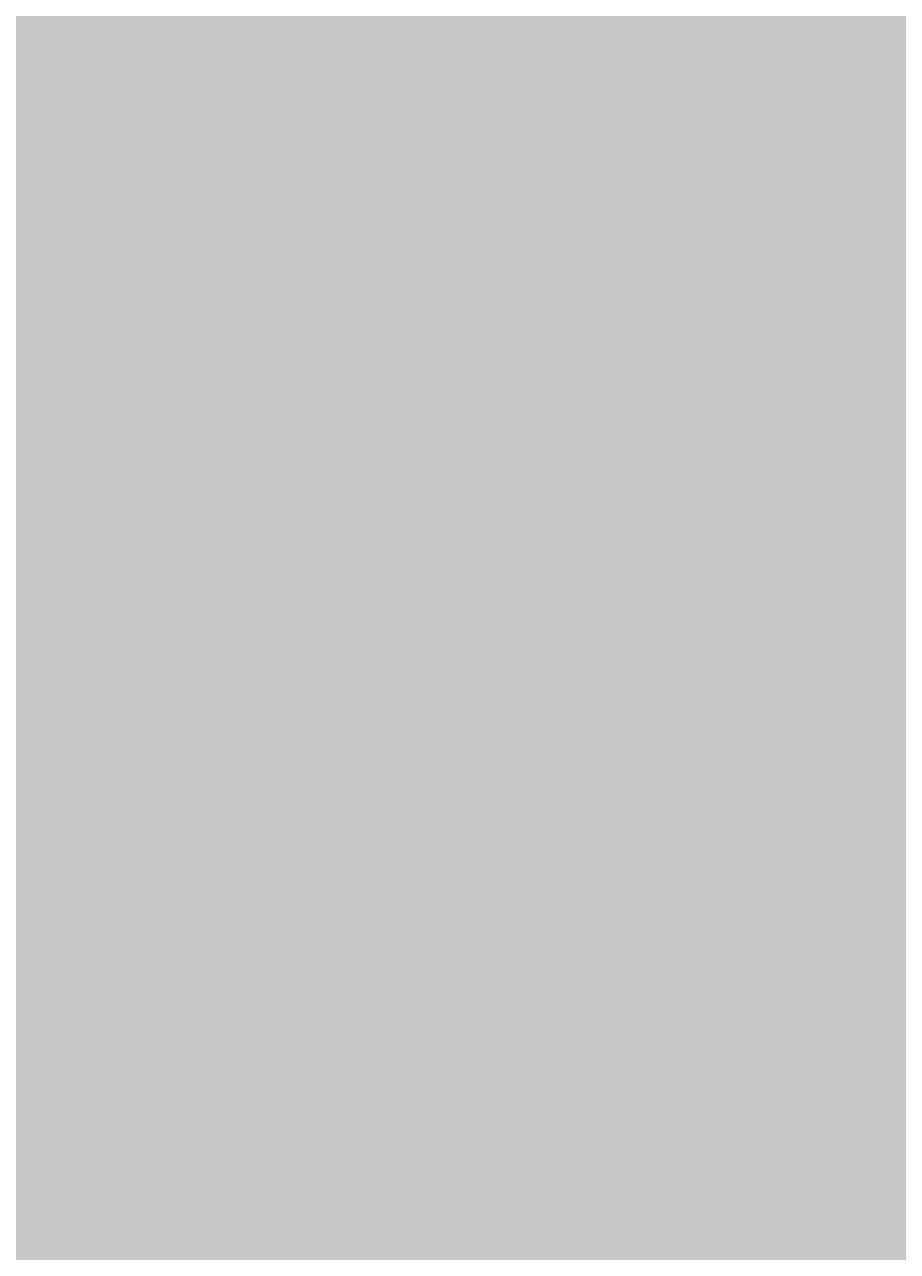
# Model space of a CAD drawing. Units: millimetres. Extents: x -22994 to 29398, y -19990 to 20176.
# Tile 106 of 135: x 216 to 237, y 95 to 124. Entities that reach past the tile are written whole.
import ezdxf

# ---------------------------------------------------------------- set-up
doc = ezdxf.new("R2010")
doc.units = ezdxf.units.MM
doc.header["$MEASUREMENT"] = 0
doc.layers.add('M-DIMS', color=2, linetype='Continuous', lineweight=18)
doc.styles.get("Standard").update_dxf_attribs({"font": 'arial.ttf'})
doc.dimstyles.get("Standard").update_dxf_attribs({"dimtxt": 0.18, "dimasz": 10000, "dimexe": 0.18, "dimexo": 0.0625, "dimgap": 0.09, "dimtad": 0, "dimtih": 1, "dimtoh": 1, "dimdec": 0, "dimzin": 0, "dimdsep": 46, "dimtxsty": 'Standard', "dimcen": 0.09, "dimadec": 0, "dimazin": 0, "dimtfac": 1, "dimtdec": 0, "dimtofl": 0, "dimtmove": 0, "dimatfit": 3, "dimfxl": 1, "dimtolj": 1, "dimtzin": 0, "dimlwd": 30, "dimarcsym": 0})

# ---------------------------------------------------------------- blocks, each defined once
blk = doc.blocks.new('*D2')
at = {"layer": 'Defpoints', "color": 0, "transparency": 16777216}
for p in [(6.677, 10.271), (290.852, 10.271), (290.852, -5.079)]:
    blk.add_point(p, dxfattribs=at)
at = {"layer": 'M-DIMS', "color": 0, "lineweight": -2, "transparency": 16777216}
for p, q in [((6.677, 10.209), (6.677, -5.259)), ((290.852, 10.209), (290.852, -5.259))]:
    blk.add_line(p, q, dxfattribs=at)
at = {"layer": 'M-DIMS', "color": 0, "lineweight": 30, "transparency": 16777216}
for p, q in [((-9993.323, -5.079), (-19993.323, -5.079)), ((10290.852, -5.079), (20290.852, -5.079))]:
    blk.add_line(p, q, dxfattribs=at)
at = {"layer": 'M-DIMS', "color": 0, "transparency": 16777216}
for points in [[(-9993.323, 1661.588), (-9993.323, -1671.745), (6.677, -5.079)], [(10290.852, 1661.588), (10290.852, -1671.745), (290.852, -5.079)]]:
    blk.add_solid(points, dxfattribs=at)
at = {"layer": 'M-DIMS', "color": 0, "transparency": 16777216, "insert": (148.765, -5.079), "char_height": 0.18, "attachment_point": 5}
blk.add_mtext('\\A1;284.2', dxfattribs=at)
blk = doc.blocks.new('*D3')
at = {"layer": 'Defpoints', "color": 0, "transparency": 16777216}
for p in [(110.265, 204.165), (110.265, 176.366), (95.833, 127.967)]:
    blk.add_point(p, dxfattribs=at)
at = {"layer": 'M-DIMS', "color": 0, "lineweight": -2, "transparency": 16777216}
for p, q in [((95.833, 128.03), (95.833, 204.345)), ((110.265, 176.429), (110.265, 204.345))]:
    blk.add_line(p, q, dxfattribs=at)
at = {"layer": 'M-DIMS', "color": 0, "lineweight": 30, "transparency": 16777216}
for p, q in [((-9904.167, 204.165), (-19904.167, 204.165)), ((10110.265, 204.165), (20110.265, 204.165))]:
    blk.add_line(p, q, dxfattribs=at)
at = {"layer": 'M-DIMS', "color": 0, "transparency": 16777216}
for points in [[(-9904.167, 1870.832), (-9904.167, -1462.501), (95.833, 204.165)], [(10110.265, 1870.832), (10110.265, -1462.501), (110.265, 204.165)]]:
    blk.add_solid(points, dxfattribs=at)
at = {"layer": 'M-DIMS', "color": 0, "transparency": 16777216, "insert": (103.049, 204.165), "char_height": 0.18, "attachment_point": 5}
blk.add_mtext('\\A1;14.432', dxfattribs=at)
blk = doc.blocks.new('*D4')
at = {"layer": 'Defpoints', "color": 0, "transparency": 16777216}
for p in [(116.265, 204.165), (110.265, 176.366), (116.265, 176.366)]:
    blk.add_point(p, dxfattribs=at)
at = {"layer": 'M-DIMS', "color": 0, "lineweight": -2, "transparency": 16777216}
for p, q in [((110.265, 176.429), (110.265, 204.345)), ((116.265, 176.429), (116.265, 204.345))]:
    blk.add_line(p, q, dxfattribs=at)
at = {"layer": 'M-DIMS', "color": 0, "lineweight": 30, "transparency": 16777216}
for p, q in [((-9889.735, 204.165), (-19889.735, 204.165)), ((10116.265, 204.165), (20116.265, 204.165))]:
    blk.add_line(p, q, dxfattribs=at)
at = {"layer": 'M-DIMS', "color": 0, "transparency": 16777216}
for points in [[(-9889.735, 1870.832), (-9889.735, -1462.501), (110.265, 204.165)], [(10116.265, 1870.832), (10116.265, -1462.501), (116.265, 204.165)]]:
    blk.add_solid(points, dxfattribs=at)
at = {"layer": 'M-DIMS', "color": 0, "transparency": 16777216, "insert": (113.265, 204.165), "char_height": 0.18, "attachment_point": 5}
blk.add_mtext('\\A1;6', dxfattribs=at)
blk = doc.blocks.new('*D5')
at = {"layer": 'Defpoints', "color": 0, "transparency": 16777216}
for p in [(181.265, 204.165), (116.265, 176.366), (181.265, 176.366)]:
    blk.add_point(p, dxfattribs=at)
at = {"layer": 'M-DIMS', "color": 0, "lineweight": -2, "transparency": 16777216}
for p, q in [((116.265, 176.429), (116.265, 204.345)), ((181.265, 176.429), (181.265, 204.345))]:
    blk.add_line(p, q, dxfattribs=at)
at = {"layer": 'M-DIMS', "color": 0, "lineweight": 30, "transparency": 16777216}
for p, q in [((-9883.735, 204.165), (-19883.735, 204.165)), ((10181.265, 204.165), (20181.265, 204.165))]:
    blk.add_line(p, q, dxfattribs=at)
at = {"layer": 'M-DIMS', "color": 0, "transparency": 16777216}
for points in [[(-9883.735, 1870.832), (-9883.735, -1462.501), (116.265, 204.165)], [(10181.265, 1870.832), (10181.265, -1462.501), (181.265, 204.165)]]:
    blk.add_solid(points, dxfattribs=at)
at = {"layer": 'M-DIMS', "color": 0, "transparency": 16777216, "insert": (148.765, 204.165), "char_height": 0.18, "attachment_point": 5}
blk.add_mtext('\\A1;65', dxfattribs=at)
blk = doc.blocks.new('*D6')
at = {"layer": 'Defpoints', "color": 0, "transparency": 16777216}
for p in [(187.265, 204.165), (181.265, 176.366), (187.265, 176.366)]:
    blk.add_point(p, dxfattribs=at)
at = {"layer": 'M-DIMS', "color": 0, "lineweight": -2, "transparency": 16777216}
for p, q in [((181.265, 176.429), (181.265, 204.345)), ((187.265, 176.429), (187.265, 204.345))]:
    blk.add_line(p, q, dxfattribs=at)
at = {"layer": 'M-DIMS', "color": 0, "lineweight": 30, "transparency": 16777216}
for p, q in [((-9818.735, 204.165), (-19818.735, 204.165)), ((10187.265, 204.165), (20187.265, 204.165))]:
    blk.add_line(p, q, dxfattribs=at)
at = {"layer": 'M-DIMS', "color": 0, "transparency": 16777216}
for points in [[(-9818.735, 1870.832), (-9818.735, -1462.501), (181.265, 204.165)], [(10187.265, 1870.832), (10187.265, -1462.501), (187.265, 204.165)]]:
    blk.add_solid(points, dxfattribs=at)
at = {"layer": 'M-DIMS', "color": 0, "transparency": 16777216, "insert": (184.265, 204.165), "char_height": 0.18, "attachment_point": 5}
blk.add_mtext('\\A1;6', dxfattribs=at)
blk = doc.blocks.new('*D7')
at = {"layer": 'Defpoints', "color": 0, "transparency": 16777216}
for p in [(201.697, 204.165), (187.265, 176.366), (201.697, 127.967)]:
    blk.add_point(p, dxfattribs=at)
at = {"layer": 'M-DIMS', "color": 0, "lineweight": -2, "transparency": 16777216}
for p, q in [((187.265, 176.429), (187.265, 204.345)), ((201.697, 128.03), (201.697, 204.345))]:
    blk.add_line(p, q, dxfattribs=at)
at = {"layer": 'M-DIMS', "color": 0, "lineweight": 30, "transparency": 16777216}
for p, q in [((-9812.735, 204.165), (-19812.735, 204.165)), ((10201.697, 204.165), (20201.697, 204.165))]:
    blk.add_line(p, q, dxfattribs=at)
at = {"layer": 'M-DIMS', "color": 0, "transparency": 16777216}
for points in [[(-9812.735, 1870.832), (-9812.735, -1462.501), (187.265, 204.165)], [(10201.697, 1870.832), (10201.697, -1462.501), (201.697, 204.165)]]:
    blk.add_solid(points, dxfattribs=at)
at = {"layer": 'M-DIMS', "color": 0, "transparency": 16777216, "insert": (194.481, 204.165), "char_height": 0.18, "attachment_point": 5}
blk.add_mtext('\\A1;14.432', dxfattribs=at)
blk = doc.blocks.new('*D8')
at = {"layer": 'Defpoints', "color": 0, "transparency": 16777216}
for p in [(227.648, 204.165), (227.648, 146.73), (201.697, 127.967)]:
    blk.add_point(p, dxfattribs=at)
at = {"layer": 'M-DIMS', "color": 0, "lineweight": -2, "transparency": 16777216}
for p, q in [((201.697, 128.03), (201.697, 204.345)), ((227.648, 146.792), (227.648, 204.345))]:
    blk.add_line(p, q, dxfattribs=at)
at = {"layer": 'M-DIMS', "color": 0, "lineweight": 30, "transparency": 16777216}
for p, q in [((-9798.303, 204.165), (-19798.303, 204.165)), ((10227.648, 204.165), (20227.648, 204.165))]:
    blk.add_line(p, q, dxfattribs=at)
at = {"layer": 'M-DIMS', "color": 0, "transparency": 16777216}
for points in [[(-9798.303, 1870.832), (-9798.303, -1462.501), (201.697, 204.165)], [(10227.648, 1870.832), (10227.648, -1462.501), (227.648, 204.165)]]:
    blk.add_solid(points, dxfattribs=at)
at = {"layer": 'M-DIMS', "color": 0, "transparency": 16777216, "insert": (214.673, 204.165), "char_height": 0.18, "attachment_point": 5}
blk.add_mtext('\\A1;25.95', dxfattribs=at)
blk = doc.blocks.new('*D9')
at = {"layer": 'Defpoints', "color": 0, "transparency": 16777216}
for p in [(187.265, 176.366), (306.202, 176.366), (290.852, 10.271)]:
    blk.add_point(p, dxfattribs=at)
at = {"layer": 'M-DIMS', "color": 0, "lineweight": 30, "transparency": 16777216}
for p, q in [((306.202, 10176.366), (306.202, 20176.366)), ((306.202, -9989.729), (306.202, -19989.729))]:
    blk.add_line(p, q, dxfattribs=at)
at = {"layer": 'M-DIMS', "color": 0, "lineweight": -2, "transparency": 16777216}
for p, q in [((187.327, 176.366), (306.382, 176.366)), ((290.915, 10.271), (306.382, 10.271))]:
    blk.add_line(p, q, dxfattribs=at)
at = {"layer": 'M-DIMS', "color": 0, "transparency": 16777216}
for points in [[(-1360.465, 10176.366), (1972.869, 10176.366), (306.202, 176.366)], [(-1360.465, -9989.729), (1972.869, -9989.729), (306.202, 10.271)]]:
    blk.add_solid(points, dxfattribs=at)
at = {"layer": 'M-DIMS', "color": 0, "transparency": 16777216, "insert": (306.202, 93.319), "char_height": 0.18, "attachment_point": 5}
blk.add_mtext('\\A1;166.1', dxfattribs=at)
blk = doc.blocks.new('*D10')
at = {"layer": 'Defpoints', "color": 0, "transparency": 16777216}
for p in [(125.65, 136.071), (133.346, 136.071), (133.346, -5.079)]:
    blk.add_point(p, dxfattribs=at)
at = {"layer": 'M-DIMS', "color": 0, "lineweight": -2, "transparency": 16777216}
for p, q in [((125.65, 136.009), (125.65, -5.259)), ((133.346, 136.009), (133.346, -5.259))]:
    blk.add_line(p, q, dxfattribs=at)
at = {"layer": 'M-DIMS', "color": 0, "lineweight": 30, "transparency": 16777216}
for p, q in [((-9874.35, -5.079), (-19874.35, -5.079)), ((10133.346, -5.079), (20133.346, -5.079))]:
    blk.add_line(p, q, dxfattribs=at)
at = {"layer": 'M-DIMS', "color": 0, "transparency": 16777216}
for points in [[(-9874.35, 1661.588), (-9874.35, -1671.745), (125.65, -5.079)], [(10133.346, 1661.588), (10133.346, -1671.745), (133.346, -5.079)]]:
    blk.add_solid(points, dxfattribs=at)
at = {"layer": 'M-DIMS', "color": 0, "transparency": 16777216, "insert": (129.498, -5.079), "char_height": 0.18, "attachment_point": 5}
blk.add_mtext('\\A1;7.696', dxfattribs=at)
blk = doc.blocks.new('*D11')
at = {"layer": 'Defpoints', "color": 0, "transparency": 16777216}
for p in [(133.346, 136.071), (135.65, 136.071), (135.65, -5.079)]:
    blk.add_point(p, dxfattribs=at)
at = {"layer": 'M-DIMS', "color": 0, "lineweight": -2, "transparency": 16777216}
for p, q in [((133.346, 136.009), (133.346, -5.259)), ((135.65, 136.009), (135.65, -5.259))]:
    blk.add_line(p, q, dxfattribs=at)
at = {"layer": 'M-DIMS', "color": 0, "lineweight": 30, "transparency": 16777216}
for p, q in [((-9866.654, -5.079), (-19866.654, -5.079)), ((10135.65, -5.079), (20135.65, -5.079))]:
    blk.add_line(p, q, dxfattribs=at)
at = {"layer": 'M-DIMS', "color": 0, "transparency": 16777216}
for points in [[(-9866.654, 1661.588), (-9866.654, -1671.745), (133.346, -5.079)], [(10135.65, 1661.588), (10135.65, -1671.745), (135.65, -5.079)]]:
    blk.add_solid(points, dxfattribs=at)
at = {"layer": 'M-DIMS', "color": 0, "transparency": 16777216, "insert": (134.498, -5.079), "char_height": 0.18, "attachment_point": 5}
blk.add_mtext('\\A1;2.304', dxfattribs=at)
blk = doc.blocks.new('*D12')
at = {"layer": 'Defpoints', "color": 0, "transparency": 16777216}
for p in [(135.65, 136.071), (145.65, 136.071), (145.65, -5.079)]:
    blk.add_point(p, dxfattribs=at)
at = {"layer": 'M-DIMS', "color": 0, "lineweight": -2, "transparency": 16777216}
for p, q in [((135.65, 136.009), (135.65, -5.259)), ((145.65, 136.009), (145.65, -5.259))]:
    blk.add_line(p, q, dxfattribs=at)
at = {"layer": 'M-DIMS', "color": 0, "lineweight": 30, "transparency": 16777216}
for p, q in [((-9864.35, -5.079), (-19864.35, -5.079)), ((10145.65, -5.079), (20145.65, -5.079))]:
    blk.add_line(p, q, dxfattribs=at)
at = {"layer": 'M-DIMS', "color": 0, "transparency": 16777216}
for points in [[(-9864.35, 1661.588), (-9864.35, -1671.745), (135.65, -5.079)], [(10145.65, 1661.588), (10145.65, -1671.745), (145.65, -5.079)]]:
    blk.add_solid(points, dxfattribs=at)
at = {"layer": 'M-DIMS', "color": 0, "transparency": 16777216, "insert": (140.65, -5.079), "char_height": 0.18, "attachment_point": 5}
blk.add_mtext('\\A1;10', dxfattribs=at)
blk = doc.blocks.new('*D13')
at = {"layer": 'Defpoints', "color": 0, "transparency": 16777216}
for p in [(145.65, 136.071), (155.65, 136.071), (155.65, -5.079)]:
    blk.add_point(p, dxfattribs=at)
at = {"layer": 'M-DIMS', "color": 0, "lineweight": -2, "transparency": 16777216}
for p, q in [((145.65, 136.009), (145.65, -5.259)), ((155.65, 136.009), (155.65, -5.259))]:
    blk.add_line(p, q, dxfattribs=at)
at = {"layer": 'M-DIMS', "color": 0, "lineweight": 30, "transparency": 16777216}
for p, q in [((-9854.35, -5.079), (-19854.35, -5.079)), ((10155.65, -5.079), (20155.65, -5.079))]:
    blk.add_line(p, q, dxfattribs=at)
at = {"layer": 'M-DIMS', "color": 0, "transparency": 16777216}
for points in [[(-9854.35, 1661.588), (-9854.35, -1671.745), (145.65, -5.079)], [(10155.65, 1661.588), (10155.65, -1671.745), (155.65, -5.079)]]:
    blk.add_solid(points, dxfattribs=at)
at = {"layer": 'M-DIMS', "color": 0, "transparency": 16777216, "insert": (150.65, -5.079), "char_height": 0.18, "attachment_point": 5}
blk.add_mtext('\\A1;10', dxfattribs=at)
blk = doc.blocks.new('*D14')
at = {"layer": 'Defpoints', "color": 0, "transparency": 16777216}
for p in [(155.65, 136.071), (165.65, 136.071), (165.65, -5.079)]:
    blk.add_point(p, dxfattribs=at)
at = {"layer": 'M-DIMS', "color": 0, "lineweight": -2, "transparency": 16777216}
for p, q in [((155.65, 136.009), (155.65, -5.259)), ((165.65, 136.009), (165.65, -5.259))]:
    blk.add_line(p, q, dxfattribs=at)
at = {"layer": 'M-DIMS', "color": 0, "lineweight": 30, "transparency": 16777216}
for p, q in [((-9844.35, -5.079), (-19844.35, -5.079)), ((10165.65, -5.079), (20165.65, -5.079))]:
    blk.add_line(p, q, dxfattribs=at)
at = {"layer": 'M-DIMS', "color": 0, "transparency": 16777216}
for points in [[(-9844.35, 1661.588), (-9844.35, -1671.745), (155.65, -5.079)], [(10165.65, 1661.588), (10165.65, -1671.745), (165.65, -5.079)]]:
    blk.add_solid(points, dxfattribs=at)
at = {"layer": 'M-DIMS', "color": 0, "transparency": 16777216, "insert": (160.65, -5.079), "char_height": 0.18, "attachment_point": 5}
blk.add_mtext('\\A1;10', dxfattribs=at)
blk = doc.blocks.new('*D15')
at = {"layer": 'Defpoints', "color": 0, "transparency": 16777216}
for p in [(173.346, 154.788), (173.346, 136.071), (306.202, 136.071)]:
    blk.add_point(p, dxfattribs=at)
at = {"layer": 'M-DIMS', "color": 0, "lineweight": 30, "transparency": 16777216}
for p, q in [((306.202, 10154.788), (306.202, 20154.788)), ((306.202, -9863.929), (306.202, -19863.929))]:
    blk.add_line(p, q, dxfattribs=at)
at = {"layer": 'M-DIMS', "color": 0, "lineweight": -2, "transparency": 16777216}
for p, q in [((173.408, 154.788), (306.382, 154.788)), ((173.408, 136.071), (306.382, 136.071))]:
    blk.add_line(p, q, dxfattribs=at)
at = {"layer": 'M-DIMS', "color": 0, "transparency": 16777216}
for points in [[(-1360.465, 10154.788), (1972.869, 10154.788), (306.202, 154.788)], [(-1360.465, -9863.929), (1972.869, -9863.929), (306.202, 136.071)]]:
    blk.add_solid(points, dxfattribs=at)
at = {"layer": 'M-DIMS', "color": 0, "transparency": 16777216, "insert": (306.202, 145.43), "char_height": 0.18, "attachment_point": 5}
blk.add_mtext('\\A1;18.717', dxfattribs=at)
blk = doc.blocks.new('*D16')
at = {"layer": 'Defpoints', "color": 0, "transparency": 16777216}
for p in [(120.17, 204.165), (110.466, 48.035), (120.17, 48.035)]:
    blk.add_point(p, dxfattribs=at)
at = {"layer": 'M-DIMS', "color": 0, "lineweight": -2, "transparency": 16777216}
for p, q in [((110.466, 48.097), (110.466, 204.345)), ((120.17, 48.097), (120.17, 204.345))]:
    blk.add_line(p, q, dxfattribs=at)
at = {"layer": 'M-DIMS', "color": 0, "lineweight": 30, "transparency": 16777216}
for p, q in [((-9889.534, 204.165), (-19889.534, 204.165)), ((10120.17, 204.165), (20120.17, 204.165))]:
    blk.add_line(p, q, dxfattribs=at)
at = {"layer": 'M-DIMS', "color": 0, "transparency": 16777216}
for points in [[(-9889.534, 1870.832), (-9889.534, -1462.501), (110.466, 204.165)], [(10120.17, 1870.832), (10120.17, -1462.501), (120.17, 204.165)]]:
    blk.add_solid(points, dxfattribs=at)
at = {"layer": 'M-DIMS', "color": 0, "transparency": 16777216, "insert": (115.318, 204.165), "char_height": 0.18, "attachment_point": 5}
blk.add_mtext('\\A1;9.704', dxfattribs=at)
blk = doc.blocks.new('*D17')
at = {"layer": 'Defpoints', "color": 0, "transparency": 16777216}
for p in [(126.17, 204.165), (120.17, 48.035), (126.17, 48.035)]:
    blk.add_point(p, dxfattribs=at)
at = {"layer": 'M-DIMS', "color": 0, "lineweight": -2, "transparency": 16777216}
for p, q in [((120.17, 48.097), (120.17, 204.345)), ((126.17, 48.097), (126.17, 204.345))]:
    blk.add_line(p, q, dxfattribs=at)
at = {"layer": 'M-DIMS', "color": 0, "lineweight": 30, "transparency": 16777216}
for p, q in [((-9879.83, 204.165), (-19879.83, 204.165)), ((10126.17, 204.165), (20126.17, 204.165))]:
    blk.add_line(p, q, dxfattribs=at)
at = {"layer": 'M-DIMS', "color": 0, "transparency": 16777216}
for points in [[(-9879.83, 1870.832), (-9879.83, -1462.501), (120.17, 204.165)], [(10126.17, 1870.832), (10126.17, -1462.501), (126.17, 204.165)]]:
    blk.add_solid(points, dxfattribs=at)
at = {"layer": 'M-DIMS', "color": 0, "transparency": 16777216, "insert": (123.17, 204.165), "char_height": 0.18, "attachment_point": 5}
blk.add_mtext('\\A1;6', dxfattribs=at)
blk = doc.blocks.new('*D18')
at = {"layer": 'Defpoints', "color": 0, "transparency": 16777216}
for p in [(132.17, 204.165), (126.17, 48.035), (132.17, 48.035)]:
    blk.add_point(p, dxfattribs=at)
at = {"layer": 'M-DIMS', "color": 0, "lineweight": -2, "transparency": 16777216}
for p, q in [((126.17, 48.097), (126.17, 204.345)), ((132.17, 48.097), (132.17, 204.345))]:
    blk.add_line(p, q, dxfattribs=at)
at = {"layer": 'M-DIMS', "color": 0, "lineweight": 30, "transparency": 16777216}
for p, q in [((-9873.83, 204.165), (-19873.83, 204.165)), ((10132.17, 204.165), (20132.17, 204.165))]:
    blk.add_line(p, q, dxfattribs=at)
at = {"layer": 'M-DIMS', "color": 0, "transparency": 16777216}
for points in [[(-9873.83, 1870.832), (-9873.83, -1462.501), (126.17, 204.165)], [(10132.17, 1870.832), (10132.17, -1462.501), (132.17, 204.165)]]:
    blk.add_solid(points, dxfattribs=at)
at = {"layer": 'M-DIMS', "color": 0, "transparency": 16777216, "insert": (129.17, 204.165), "char_height": 0.18, "attachment_point": 5}
blk.add_mtext('\\A1;6', dxfattribs=at)
blk = doc.blocks.new('*D19')
at = {"layer": 'Defpoints', "color": 0, "transparency": 16777216}
for p in [(138.17, 204.165), (132.17, 48.035), (138.17, 48.035)]:
    blk.add_point(p, dxfattribs=at)
at = {"layer": 'M-DIMS', "color": 0, "lineweight": -2, "transparency": 16777216}
for p, q in [((132.17, 48.097), (132.17, 204.345)), ((138.17, 48.097), (138.17, 204.345))]:
    blk.add_line(p, q, dxfattribs=at)
at = {"layer": 'M-DIMS', "color": 0, "lineweight": 30, "transparency": 16777216}
for p, q in [((-9867.83, 204.165), (-19867.83, 204.165)), ((10138.17, 204.165), (20138.17, 204.165))]:
    blk.add_line(p, q, dxfattribs=at)
at = {"layer": 'M-DIMS', "color": 0, "transparency": 16777216}
for points in [[(-9867.83, 1870.832), (-9867.83, -1462.501), (132.17, 204.165)], [(10138.17, 1870.832), (10138.17, -1462.501), (138.17, 204.165)]]:
    blk.add_solid(points, dxfattribs=at)
at = {"layer": 'M-DIMS', "color": 0, "transparency": 16777216, "insert": (135.17, 204.165), "char_height": 0.18, "attachment_point": 5}
blk.add_mtext('\\A1;6', dxfattribs=at)
blk = doc.blocks.new('*D20')
at = {"layer": 'Defpoints', "color": 0, "transparency": 16777216}
for p in [(144.17, 204.165), (138.17, 48.035), (144.17, 48.035)]:
    blk.add_point(p, dxfattribs=at)
at = {"layer": 'M-DIMS', "color": 0, "lineweight": -2, "transparency": 16777216}
for p, q in [((138.17, 48.097), (138.17, 204.345)), ((144.17, 48.097), (144.17, 204.345))]:
    blk.add_line(p, q, dxfattribs=at)
at = {"layer": 'M-DIMS', "color": 0, "lineweight": 30, "transparency": 16777216}
for p, q in [((-9861.83, 204.165), (-19861.83, 204.165)), ((10144.17, 204.165), (20144.17, 204.165))]:
    blk.add_line(p, q, dxfattribs=at)
at = {"layer": 'M-DIMS', "color": 0, "transparency": 16777216}
for points in [[(-9861.83, 1870.832), (-9861.83, -1462.501), (138.17, 204.165)], [(10144.17, 1870.832), (10144.17, -1462.501), (144.17, 204.165)]]:
    blk.add_solid(points, dxfattribs=at)
at = {"layer": 'M-DIMS', "color": 0, "transparency": 16777216, "insert": (141.17, 204.165), "char_height": 0.18, "attachment_point": 5}
blk.add_mtext('\\A1;6', dxfattribs=at)
blk = doc.blocks.new('*D21')
at = {"layer": 'Defpoints', "color": 0, "transparency": 16777216}
for p in [(149.116, 204.165), (144.17, 48.035), (149.116, 48.035)]:
    blk.add_point(p, dxfattribs=at)
at = {"layer": 'M-DIMS', "color": 0, "lineweight": -2, "transparency": 16777216}
for p, q in [((144.17, 48.097), (144.17, 204.345)), ((149.116, 48.097), (149.116, 204.345))]:
    blk.add_line(p, q, dxfattribs=at)
at = {"layer": 'M-DIMS', "color": 0, "lineweight": 30, "transparency": 16777216}
for p, q in [((-9855.83, 204.165), (-19855.83, 204.165)), ((10149.116, 204.165), (20149.116, 204.165))]:
    blk.add_line(p, q, dxfattribs=at)
at = {"layer": 'M-DIMS', "color": 0, "transparency": 16777216}
for points in [[(-9855.83, 1870.832), (-9855.83, -1462.501), (144.17, 204.165)], [(10149.116, 1870.832), (10149.116, -1462.501), (149.116, 204.165)]]:
    blk.add_solid(points, dxfattribs=at)
at = {"layer": 'M-DIMS', "color": 0, "transparency": 16777216, "insert": (146.643, 204.165), "char_height": 0.18, "attachment_point": 5}
blk.add_mtext('\\A1;4.945', dxfattribs=at)
blk = doc.blocks.new('*D22')
at = {"layer": 'Defpoints', "color": 0, "transparency": 16777216}
for p in [(149.116, 30.99), (155.116, 30.99), (155.116, -5.079)]:
    blk.add_point(p, dxfattribs=at)
at = {"layer": 'M-DIMS', "color": 0, "lineweight": -2, "transparency": 16777216}
for p, q in [((149.116, 30.927), (149.116, -5.259)), ((155.116, 30.927), (155.116, -5.259))]:
    blk.add_line(p, q, dxfattribs=at)
at = {"layer": 'M-DIMS', "color": 0, "lineweight": 30, "transparency": 16777216}
for p, q in [((-9850.884, -5.079), (-19850.884, -5.079)), ((10155.116, -5.079), (20155.116, -5.079))]:
    blk.add_line(p, q, dxfattribs=at)
at = {"layer": 'M-DIMS', "color": 0, "transparency": 16777216}
for points in [[(-9850.884, 1661.588), (-9850.884, -1671.745), (149.116, -5.079)], [(10155.116, 1661.588), (10155.116, -1671.745), (155.116, -5.079)]]:
    blk.add_solid(points, dxfattribs=at)
at = {"layer": 'M-DIMS', "color": 0, "transparency": 16777216, "insert": (152.116, -5.079), "char_height": 0.18, "attachment_point": 5}
blk.add_mtext('\\A1;6', dxfattribs=at)
blk = doc.blocks.new('*D23')
at = {"layer": 'Defpoints', "color": 0, "transparency": 16777216}
for p in [(155.116, 30.99), (161.116, 30.99), (161.116, -5.079)]:
    blk.add_point(p, dxfattribs=at)
at = {"layer": 'M-DIMS', "color": 0, "lineweight": -2, "transparency": 16777216}
for p, q in [((155.116, 30.927), (155.116, -5.259)), ((161.116, 30.927), (161.116, -5.259))]:
    blk.add_line(p, q, dxfattribs=at)
at = {"layer": 'M-DIMS', "color": 0, "lineweight": 30, "transparency": 16777216}
for p, q in [((-9844.884, -5.079), (-19844.884, -5.079)), ((10161.116, -5.079), (20161.116, -5.079))]:
    blk.add_line(p, q, dxfattribs=at)
at = {"layer": 'M-DIMS', "color": 0, "transparency": 16777216}
for points in [[(-9844.884, 1661.588), (-9844.884, -1671.745), (155.116, -5.079)], [(10161.116, 1661.588), (10161.116, -1671.745), (161.116, -5.079)]]:
    blk.add_solid(points, dxfattribs=at)
at = {"layer": 'M-DIMS', "color": 0, "transparency": 16777216, "insert": (158.116, -5.079), "char_height": 0.18, "attachment_point": 5}
blk.add_mtext('\\A1;6', dxfattribs=at)
blk = doc.blocks.new('*D24')
at = {"layer": 'Defpoints', "color": 0, "transparency": 16777216}
for p in [(161.116, 30.99), (166.439, 30.99), (166.439, -5.079)]:
    blk.add_point(p, dxfattribs=at)
at = {"layer": 'M-DIMS', "color": 0, "lineweight": -2, "transparency": 16777216}
for p, q in [((161.116, 30.927), (161.116, -5.259)), ((166.439, 30.927), (166.439, -5.259))]:
    blk.add_line(p, q, dxfattribs=at)
at = {"layer": 'M-DIMS', "color": 0, "lineweight": 30, "transparency": 16777216}
for p, q in [((-9838.884, -5.079), (-19838.884, -5.079)), ((10166.439, -5.079), (20166.439, -5.079))]:
    blk.add_line(p, q, dxfattribs=at)
at = {"layer": 'M-DIMS', "color": 0, "transparency": 16777216}
for points in [[(-9838.884, 1661.588), (-9838.884, -1671.745), (161.116, -5.079)], [(10166.439, 1661.588), (10166.439, -1671.745), (166.439, -5.079)]]:
    blk.add_solid(points, dxfattribs=at)
at = {"layer": 'M-DIMS', "color": 0, "transparency": 16777216, "insert": (163.777, -5.079), "char_height": 0.18, "attachment_point": 5}
blk.add_mtext('\\A1;5.323', dxfattribs=at)
blk = doc.blocks.new('*D25')
at = {"layer": 'Defpoints', "color": 0, "transparency": 16777216}
for p in [(166.439, 30.99), (172.439, 30.99), (172.439, -5.079)]:
    blk.add_point(p, dxfattribs=at)
at = {"layer": 'M-DIMS', "color": 0, "lineweight": -2, "transparency": 16777216}
for p, q in [((166.439, 30.927), (166.439, -5.259)), ((172.439, 30.927), (172.439, -5.259))]:
    blk.add_line(p, q, dxfattribs=at)
at = {"layer": 'M-DIMS', "color": 0, "lineweight": 30, "transparency": 16777216}
for p, q in [((-9833.561, -5.079), (-19833.561, -5.079)), ((10172.439, -5.079), (20172.439, -5.079))]:
    blk.add_line(p, q, dxfattribs=at)
at = {"layer": 'M-DIMS', "color": 0, "transparency": 16777216}
for points in [[(-9833.561, 1661.588), (-9833.561, -1671.745), (166.439, -5.079)], [(10172.439, 1661.588), (10172.439, -1671.745), (172.439, -5.079)]]:
    blk.add_solid(points, dxfattribs=at)
at = {"layer": 'M-DIMS', "color": 0, "transparency": 16777216, "insert": (169.439, -5.079), "char_height": 0.18, "attachment_point": 5}
blk.add_mtext('\\A1;6', dxfattribs=at)
blk = doc.blocks.new('*D26')
at = {"layer": 'Defpoints', "color": 0, "transparency": 16777216}
for p in [(172.439, 30.99), (178.439, 30.99), (178.439, -5.079)]:
    blk.add_point(p, dxfattribs=at)
at = {"layer": 'M-DIMS', "color": 0, "lineweight": -2, "transparency": 16777216}
for p, q in [((172.439, 30.927), (172.439, -5.259)), ((178.439, 30.927), (178.439, -5.259))]:
    blk.add_line(p, q, dxfattribs=at)
at = {"layer": 'M-DIMS', "color": 0, "lineweight": 30, "transparency": 16777216}
for p, q in [((-9827.561, -5.079), (-19827.561, -5.079)), ((10178.439, -5.079), (20178.439, -5.079))]:
    blk.add_line(p, q, dxfattribs=at)
at = {"layer": 'M-DIMS', "color": 0, "transparency": 16777216}
for points in [[(-9827.561, 1661.588), (-9827.561, -1671.745), (172.439, -5.079)], [(10178.439, 1661.588), (10178.439, -1671.745), (178.439, -5.079)]]:
    blk.add_solid(points, dxfattribs=at)
at = {"layer": 'M-DIMS', "color": 0, "transparency": 16777216, "insert": (175.439, -5.079), "char_height": 0.18, "attachment_point": 5}
blk.add_mtext('\\A1;6', dxfattribs=at)
blk = doc.blocks.new('*D27')
at = {"layer": 'Defpoints', "color": 0, "transparency": 16777216}
for p in [(178.439, 30.99), (188.117, 30.99), (188.117, -5.079)]:
    blk.add_point(p, dxfattribs=at)
at = {"layer": 'M-DIMS', "color": 0, "lineweight": -2, "transparency": 16777216}
for p, q in [((178.439, 30.927), (178.439, -5.259)), ((188.117, 30.927), (188.117, -5.259))]:
    blk.add_line(p, q, dxfattribs=at)
at = {"layer": 'M-DIMS', "color": 0, "lineweight": 30, "transparency": 16777216}
for p, q in [((-9821.561, -5.079), (-19821.561, -5.079)), ((10188.117, -5.079), (20188.117, -5.079))]:
    blk.add_line(p, q, dxfattribs=at)
at = {"layer": 'M-DIMS', "color": 0, "transparency": 16777216}
for points in [[(-9821.561, 1661.588), (-9821.561, -1671.745), (178.439, -5.079)], [(10188.117, 1661.588), (10188.117, -1671.745), (188.117, -5.079)]]:
    blk.add_solid(points, dxfattribs=at)
at = {"layer": 'M-DIMS', "color": 0, "transparency": 16777216, "insert": (183.278, -5.079), "char_height": 0.18, "attachment_point": 5}
blk.add_mtext('\\A1;9.679', dxfattribs=at)
blk = doc.blocks.new('*D28')
at = {"layer": 'Defpoints', "color": 0, "transparency": 16777216}
for p in [(188.117, 48.035), (306.202, 48.035), (188.117, 30.99)]:
    blk.add_point(p, dxfattribs=at)
at = {"layer": 'M-DIMS', "color": 0, "lineweight": 30, "transparency": 16777216}
for p, q in [((306.202, 10048.035), (306.202, 20048.035)), ((306.202, -9969.01), (306.202, -19969.01))]:
    blk.add_line(p, q, dxfattribs=at)
at = {"layer": 'M-DIMS', "color": 0, "lineweight": -2, "transparency": 16777216}
for p, q in [((188.18, 48.035), (306.382, 48.035)), ((188.18, 30.99), (306.382, 30.99))]:
    blk.add_line(p, q, dxfattribs=at)
at = {"layer": 'M-DIMS', "color": 0, "transparency": 16777216}
for points in [[(-1360.465, 10048.035), (1972.869, 10048.035), (306.202, 48.035)], [(-1360.465, -9969.01), (1972.869, -9969.01), (306.202, 30.99)]]:
    blk.add_solid(points, dxfattribs=at)
at = {"layer": 'M-DIMS', "color": 0, "transparency": 16777216, "insert": (306.202, 39.512), "char_height": 0.18, "attachment_point": 5}
blk.add_mtext('\\A1;17.045', dxfattribs=at)
blk = doc.blocks.new('*D29')
at = {"layer": 'Defpoints', "color": 0, "transparency": 16777216}
for p in [(36.801, 80.045), (64.03, 80.045)]:
    blk.add_point(p, dxfattribs=at)
at = {"layer": 'M-DIMS', "color": 0, "lineweight": -2, "transparency": 16777216}
for p, q in [((50.325, 80.045), (50.505, 80.045)), ((50.415, 79.955), (50.415, 80.135))]:
    blk.add_line(p, q, dxfattribs=at)
at = {"layer": 'M-DIMS', "color": 0, "lineweight": 30, "transparency": 16777216}
blk.add_line((20064.03, 80.03), (10064.03, 80.038), dxfattribs=at)
at = {"layer": 'M-DIMS', "color": 0, "transparency": 16777216}
blk.add_solid([(10064.031, 1746.704), (10064.028, -1586.629), (64.03, 80.045)], dxfattribs=at)
at = {"layer": 'M-DIMS', "color": 0, "transparency": 16777216, "insert": (20064.521, 80.03), "char_height": 0.18, "attachment_point": 5}
blk.add_mtext('\\A1;∅27.23', dxfattribs=at)
blk = doc.blocks.new('*D30')
at = {"layer": 'Defpoints', "color": 0, "transparency": 16777216}
for p in [(216.315, 146.729), (238.982, 146.73)]:
    blk.add_point(p, dxfattribs=at)
at = {"layer": 'M-DIMS', "color": 0, "lineweight": 30, "transparency": 16777216}
blk.add_line((20238.982, 147.496), (10238.982, 147.113), dxfattribs=at)
at = {"layer": 'M-DIMS', "color": 0, "lineweight": -2, "transparency": 16777216}
for p, q in [((227.558, 146.73), (227.738, 146.73)), ((227.648, 146.64), (227.648, 146.82))]:
    blk.add_line(p, q, dxfattribs=at)
at = {"layer": 'M-DIMS', "color": 0, "transparency": 16777216}
blk.add_solid([(10238.918, 1813.78), (10239.046, -1519.554), (238.982, 146.73)], dxfattribs=at)
at = {"layer": 'M-DIMS', "color": 0, "transparency": 16777216, "insert": (20239.544, 147.496), "char_height": 0.18, "attachment_point": 5}
blk.add_mtext('\\A1;∅22.667', dxfattribs=at)
blk = doc.blocks.new('*D31')
at = {"layer": 'Defpoints', "color": 0, "transparency": 16777216}
for p in [(223.164, 146.729), (232.133, 146.73)]:
    blk.add_point(p, dxfattribs=at)
at = {"layer": 'M-DIMS', "color": 0, "lineweight": 30, "transparency": 16777216}
blk.add_line((20232.133, 148.666), (10232.133, 147.698), dxfattribs=at)
at = {"layer": 'M-DIMS', "color": 0, "lineweight": -2, "transparency": 16777216}
for p, q in [((227.558, 146.73), (227.738, 146.73)), ((227.648, 146.64), (227.648, 146.82))]:
    blk.add_line(p, q, dxfattribs=at)
at = {"layer": 'M-DIMS', "color": 0, "transparency": 16777216}
blk.add_solid([(10231.971, 1814.364), (10232.294, -1518.969), (232.133, 146.73)], dxfattribs=at)
at = {"layer": 'M-DIMS', "color": 0, "transparency": 16777216, "insert": (20232.625, 148.666), "char_height": 0.18, "attachment_point": 5}
blk.add_mtext('\\A1;∅8.969', dxfattribs=at)
blk = doc.blocks.new('*D33')
at = {"layer": 'Defpoints', "color": 0, "transparency": 16777216}
for p in [(229.561, 154.377), (232.997, 153.351)]:
    blk.add_point(p, dxfattribs=at)
at = {"layer": 'M-DIMS', "color": 0, "lineweight": -2, "transparency": 16777216}
for p, q in [((229.471, 154.377), (229.651, 154.377)), ((229.561, 154.287), (229.561, 154.467))]:
    blk.add_line(p, q, dxfattribs=at)
at = {"layer": 'M-DIMS', "color": 0, "lineweight": 30, "transparency": 16777216}
for p, q in [((19396.339, -5570.838), (9814.668, -2708.743)), ((29396.339, -5570.838), (19396.339, -5570.838))]:
    blk.add_line(p, q, dxfattribs=at)
at = {"layer": 'M-DIMS', "color": 0, "transparency": 16777216}
blk.add_solid([(10291.684, -1111.798), (9337.652, -4305.689), (232.997, 153.351)], dxfattribs=at)
at = {"layer": 'M-DIMS', "color": 0, "transparency": 16777216, "insert": (29397.012, -5570.838), "char_height": 0.18, "attachment_point": 5}
blk.add_mtext('\\A1;6X R3.586', dxfattribs=at)
blk = doc.blocks.new('*D34')
at = {"layer": 'Defpoints', "color": 0, "transparency": 16777216}
for p in [(178.58, 122.895), (176.812, 121.128)]:
    blk.add_point(p, dxfattribs=at)
at = {"layer": 'M-DIMS', "color": 0, "lineweight": 30, "transparency": 16777216}
for p, q in [((14322.436, 14263.311), (7250.508, 7193.103)), ((24322.436, 14263.311), (14322.436, 14263.311))]:
    blk.add_line(p, q, dxfattribs=at)
at = {"layer": 'M-DIMS', "color": 0, "lineweight": -2, "transparency": 16777216}
for p, q in [((176.722, 121.128), (176.902, 121.128)), ((176.812, 121.038), (176.812, 121.218))]:
    blk.add_line(p, q, dxfattribs=at)
at = {"layer": 'M-DIMS', "color": 0, "transparency": 16777216}
blk.add_solid([(6072.14, 8371.758), (8428.876, 6014.448), (178.58, 122.895)], dxfattribs=at)
at = {"layer": 'M-DIMS', "color": 0, "transparency": 16777216, "insert": (24322.97, 14263.311), "char_height": 0.18, "attachment_point": 5}
blk.add_mtext('\\A1;6X R2.5', dxfattribs=at)
blk = doc.blocks.new('*D36')
at = {"layer": 'Defpoints', "color": 0, "transparency": 16777216}
for p in [(46.39, 31.303), (46.387, 26.593)]:
    blk.add_point(p, dxfattribs=at)
at = {"layer": 'M-DIMS', "color": 0, "lineweight": 30, "transparency": 16777216}
for p, q in [((57.15, 20031.301), (51.77, 10031.302)), ((10057.15, 20031.301), (57.15, 20031.301))]:
    blk.add_line(p, q, dxfattribs=at)
at = {"layer": 'M-DIMS', "color": 0, "lineweight": -2, "transparency": 16777216}
for p, q in [((46.299, 28.948), (46.479, 28.948)), ((46.389, 28.858), (46.389, 29.038))]:
    blk.add_line(p, q, dxfattribs=at)
at = {"layer": 'M-DIMS', "color": 0, "transparency": 16777216}
blk.add_solid([(-1614.896, 10032.199), (1718.436, 10030.405), (46.39, 31.303)], dxfattribs=at)
at = {"layer": 'M-DIMS', "color": 0, "transparency": 16777216, "insert": (10057.554, 20031.301), "char_height": 0.18, "attachment_point": 5}
blk.add_mtext('\\A1;∅4.71', dxfattribs=at)
blk = doc.blocks.new('*D37')
at = {"layer": 'Defpoints', "color": 0, "transparency": 16777216}
for p in [(54.834, 118.615), (59.494, 118.614)]:
    blk.add_point(p, dxfattribs=at)
at = {"layer": 'M-DIMS', "color": 0, "lineweight": -2, "transparency": 16777216}
for p, q in [((57.074, 118.614), (57.254, 118.614)), ((57.164, 118.524), (57.164, 118.704))]:
    blk.add_line(p, q, dxfattribs=at)
at = {"layer": 'M-DIMS', "color": 0, "lineweight": 30, "transparency": 16777216}
blk.add_line((20059.493, 116.253), (10059.494, 117.434), dxfattribs=at)
at = {"layer": 'M-DIMS', "color": 0, "transparency": 16777216}
blk.add_solid([(10059.69, 1784.1), (10059.297, -1549.233), (59.494, 118.614)], dxfattribs=at)
at = {"layer": 'M-DIMS', "color": 0, "transparency": 16777216, "insert": (20059.985, 116.253), "char_height": 0.18, "attachment_point": 5}
blk.add_mtext('\\A1;∅4.659', dxfattribs=at)

msp = doc.modelspace()

# ---------------------------------------------------------------- dimensions: what is measured, and where the dimension line sits
at = {"layer": 'M-DIMS'}
for base, p1, p2, override, picture, middle in [((306.202, 176.3662), (290.852, 10.2713), (187.2647, 176.3662), {"dimdec": 1, "dimlfac": 1, "dimrnd": 0, "dimzin": 0, "dimdsep": 46, "dimlunit": 2}, '*D9', (306.202, 93.3187)), ((306.202, 136.0713), (173.3459, 154.788), (173.3459, 136.0713), {"dimdec": 3, "dimlfac": 1, "dimrnd": 0, "dimzin": 0, "dimdsep": 46, "dimlunit": 2}, '*D15', (306.202, 145.4297)), ((306.202, 48.0349), (188.1175, 30.9895), (188.1175, 48.0349), {"dimdec": 3, "dimlfac": 1, "dimrnd": 0, "dimzin": 0, "dimdsep": 46, "dimlunit": 2}, '*D28', (306.202, 39.5122))]:
    dim = msp.add_linear_dim(base=base, p1=p1, p2=p2, angle=90, dimstyle='Standard', override=override, dxfattribs=at)
    dim.commit()
    dim.dimension.update_dxf_attribs({"geometry": picture, "text_midpoint": middle})
for p1, p2, override, picture, middle in [((46.3875, 26.5934), (46.39, 31.3035), {"dimdec": 2, "dimlfac": 1, "dimrnd": 0, "dimzin": 0, "dimdsep": 46, "dimlunit": 2}, '*D36', (10057.5542, 20031.3006)), ((223.1641, 146.7291), (232.1328, 146.73), {"dimdec": 3, "dimlfac": 1, "dimrnd": 0, "dimzin": 0, "dimdsep": 46, "dimlunit": 2}, '*D31', (20232.1327, 148.6656)), ((216.3148, 146.7291), (238.9821, 146.73), {"dimdec": 3, "dimlfac": 1, "dimrnd": 0, "dimzin": 0, "dimdsep": 46, "dimlunit": 2}, '*D30', (20238.9821, 147.4959))]:
    dim = msp.add_diameter_dim_2p(p1=p1, p2=p2, dimstyle='Standard', override=override, dxfattribs=at)
    dim.commit()
    dim.dimension.update_dxf_attribs({"geometry": picture, "text_midpoint": middle, "dimtype": 163})
for center, mpoint, override, picture, middle in [((176.8123, 121.1277), (178.5802, 122.8952), {"dimdec": 1, "dimlfac": 1, "dimrnd": 0, "dimzin": 0, "dimdsep": 46, "dimlunit": 2}, '*D34', (24322.9703, 14263.3108)), ((229.5613, 154.3773), (232.9972, 153.3509), {"dimdec": 3, "dimlfac": 1, "dimrnd": 0, "dimzin": 0, "dimdsep": 46, "dimlunit": 2}, '*D33', (29397.0125, -5570.8378))]:
    dim = msp.add_radius_dim(center=center, mpoint=mpoint, text='6X <>', dimstyle='Standard', override=override, dxfattribs=at)
    dim.commit()
    dim.dimension.update_dxf_attribs({"geometry": picture, "text_midpoint": middle})
for base, p1, p2, override, picture, middle in [((110.2647, 204.1654), (95.8327, 127.967), (110.2647, 176.3662), {"dimdec": 3, "dimlfac": 1, "dimrnd": 0, "dimzin": 0, "dimdsep": 46, "dimlunit": 2}, '*D3', (103.0487, 204.1654)), ((116.2647, 204.1654), (110.2647, 176.3662), (116.2647, 176.3662), {"dimdec": 0, "dimlfac": 1, "dimrnd": 0, "dimzin": 0, "dimdsep": 46, "dimlunit": 2}, '*D4', (113.2647, 204.1654)), ((120.1702, 204.1654), (110.4658, 48.0349), (120.1702, 48.0349), {"dimdec": 3, "dimlfac": 1, "dimrnd": 0, "dimzin": 0, "dimdsep": 46, "dimlunit": 2}, '*D16', (115.318, 204.1654)), ((181.2647, 204.1654), (116.2647, 176.3662), (181.2647, 176.3662), {"dimdec": 0, "dimlfac": 1, "dimrnd": 0, "dimzin": 0, "dimdsep": 46, "dimlunit": 2}, '*D5', (148.7647, 204.1654)), ((126.1702, 204.1654), (120.1702, 48.0349), (126.1702, 48.0349), {"dimdec": 0, "dimlfac": 1, "dimrnd": 0, "dimzin": 0, "dimdsep": 46, "dimlunit": 2}, '*D17', (123.1702, 204.1654)), ((132.1702, 204.1654), (126.1702, 48.0349), (132.1702, 48.0349), {"dimdec": 0, "dimlfac": 1, "dimrnd": 0, "dimzin": 0, "dimdsep": 46, "dimlunit": 2}, '*D18', (129.1702, 204.1654)), ((138.1702, 204.1654), (132.1702, 48.0349), (138.1702, 48.0349), {"dimdec": 0, "dimlfac": 1, "dimrnd": 0, "dimzin": 0, "dimdsep": 46, "dimlunit": 2}, '*D19', (135.1702, 204.1654)), ((144.1702, 204.1654), (138.1702, 48.0349), (144.1702, 48.0349), {"dimdec": 0, "dimlfac": 1, "dimrnd": 0, "dimzin": 0, "dimdsep": 46, "dimlunit": 2}, '*D20', (141.1702, 204.1654)), ((149.11567, 204.16539), (144.17023, 48.03494), (149.11567, 48.03494), {"dimdec": 3, "dimlfac": 1, "dimrnd": 0, "dimzin": 0, "dimdsep": 46, "dimlunit": 2}, '*D21', (146.64295, 204.16539)), ((187.2647, 204.1654), (181.2647, 176.3662), (187.2647, 176.3662), {"dimdec": 0, "dimlfac": 1, "dimrnd": 0, "dimzin": 0, "dimdsep": 46, "dimlunit": 2}, '*D6', (184.2647, 204.1654)), ((201.6967, 204.1654), (187.2647, 176.3662), (201.6967, 127.967), {"dimdec": 3, "dimlfac": 1, "dimrnd": 0, "dimzin": 0, "dimdsep": 46, "dimlunit": 2}, '*D7', (194.4807, 204.1654)), ((227.6485, 204.1654), (201.6967, 127.967), (227.6485, 146.7296), {"dimdec": 2, "dimlfac": 1, "dimrnd": 0, "dimzin": 0, "dimdsep": 46, "dimlunit": 2}, '*D8', (214.6726, 204.1654)), ((290.852, -5.0787), (6.6773, 10.2713), (290.852, 10.2713), {"dimdec": 1, "dimlfac": 1, "dimrnd": 0, "dimzin": 0, "dimdsep": 46, "dimlunit": 2}, '*D2', (148.7647, -5.0787)), ((133.3459, -5.0787), (125.6498, 136.0713), (133.3459, 136.0713), {"dimdec": 3, "dimlfac": 1, "dimrnd": 0, "dimzin": 0, "dimdsep": 46, "dimlunit": 2}, '*D10', (129.4978, -5.0787)), ((135.6498, -5.0787), (133.3459, 136.0713), (135.6498, 136.0713), {"dimdec": 3, "dimlfac": 1, "dimrnd": 0, "dimzin": 0, "dimdsep": 46, "dimlunit": 2}, '*D11', (134.4978, -5.0787)), ((145.6498, -5.0787), (135.6498, 136.0713), (145.6498, 136.0713), {"dimdec": 0, "dimlfac": 1, "dimrnd": 0, "dimzin": 0, "dimdsep": 46, "dimlunit": 2}, '*D12', (140.6498, -5.0787)), ((155.6498, -5.0787), (145.6498, 136.0713), (155.6498, 136.0713), {"dimdec": 0, "dimlfac": 1, "dimrnd": 0, "dimzin": 0, "dimdsep": 46, "dimlunit": 2}, '*D13', (150.6498, -5.0787)), ((155.1157, -5.0787), (149.1157, 30.9895), (155.1157, 30.9895), {"dimdec": 0, "dimlfac": 1, "dimrnd": 0, "dimzin": 0, "dimdsep": 46, "dimlunit": 2}, '*D22', (152.1157, -5.0787)), ((161.1157, -5.0787), (155.1157, 30.9895), (161.1157, 30.9895), {"dimdec": 0, "dimlfac": 1, "dimrnd": 0, "dimzin": 0, "dimdsep": 46, "dimlunit": 2}, '*D23', (158.1157, -5.0787)), ((165.6498, -5.0787), (155.6498, 136.0713), (165.6498, 136.0713), {"dimdec": 0, "dimlfac": 1, "dimrnd": 0, "dimzin": 0, "dimdsep": 46, "dimlunit": 2}, '*D14', (160.6498, -5.0787)), ((166.4387, -5.0787), (161.1157, 30.9895), (166.4387, 30.9895), {"dimdec": 3, "dimlfac": 1, "dimrnd": 0, "dimzin": 0, "dimdsep": 46, "dimlunit": 2}, '*D24', (163.7772, -5.0787)), ((172.4387, -5.0787), (166.4387, 30.9895), (172.4387, 30.9895), {"dimdec": 0, "dimlfac": 1, "dimrnd": 0, "dimzin": 0, "dimdsep": 46, "dimlunit": 2}, '*D25', (169.4387, -5.0787)), ((178.4387, -5.0787), (172.4387, 30.9895), (178.4387, 30.9895), {"dimdec": 0, "dimlfac": 1, "dimrnd": 0, "dimzin": 0, "dimdsep": 46, "dimlunit": 2}, '*D26', (175.4387, -5.0787)), ((188.1175, -5.0787), (178.4387, 30.9895), (188.1175, 30.9895), {"dimdec": 3, "dimlfac": 1, "dimrnd": 0, "dimzin": 0, "dimdsep": 46, "dimlunit": 2}, '*D27', (183.2781, -5.0787))]:
    dim = msp.add_linear_dim(base=base, p1=p1, p2=p2, dimstyle='Standard', override=override, dxfattribs=at)
    dim.commit()
    dim.dimension.update_dxf_attribs({"geometry": picture, "text_midpoint": middle})
for p1, p2, override, picture, middle in [((54.8343, 118.6145), (59.4936, 118.614), {"dimdec": 3, "dimlfac": 1, "dimrnd": 0, "dimzin": 0, "dimdsep": 46, "dimlunit": 2}, '*D37', (20059.4934, 116.2531)), ((36.8006, 80.045), (64.0296, 80.045), {"dimdec": 2, "dimlfac": 1, "dimrnd": 0, "dimzin": 0, "dimdsep": 46, "dimlunit": 2}, '*D29', (20064.0296, 80.0303))]:
    dim = msp.add_diameter_dim_2p(p1=p1, p2=p2, dimstyle='Standard', override=override, dxfattribs=at)
    dim.commit()
    dim.dimension.update_dxf_attribs({"geometry": picture, "text_midpoint": middle})

doc.saveas('drawing.dxf')
